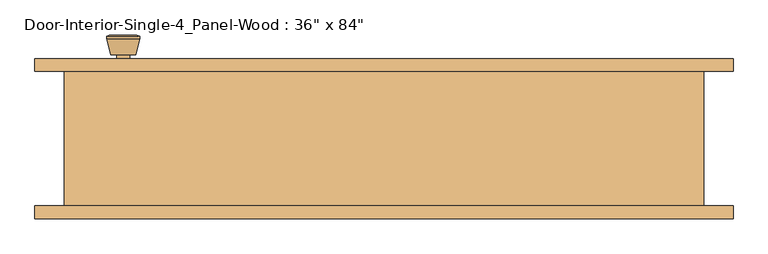
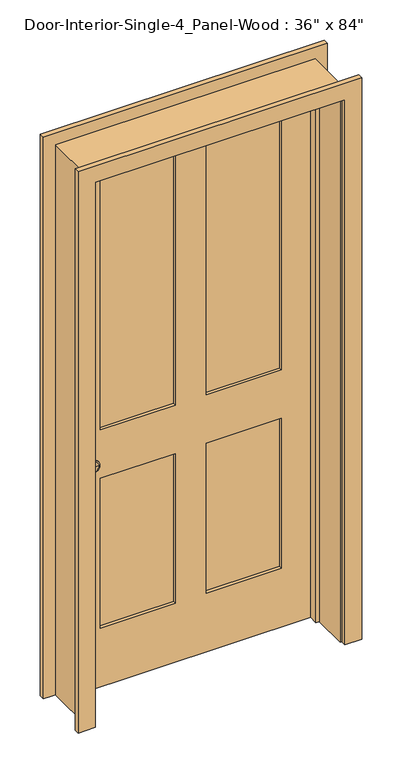
"""IFC4 building model written with IfcOpenShell, lengths in millimetres: door geometry."""

from ifc_helpers import new_model, si_unit, point, frame, frame_2d, origin, place, context, project, spatial, polyline, circle_curve, trimmed, segment, composite_curve, outline, extrude, faceted_brep, source, transform, mapped, element, save
from ifc_brep_helpers import plane_surface, cylinder_surface, revolved_surface, advanced_brep


def door_2d5c49d3(model_context):
    return source(origin(), model_context, "Body", "SolidModel", [
        advanced_brep(
        [(-393.7, 57.5, 914.4), (-383.7, 57.5, 914.4), (-403.7, 57.5, 914.4), (-373.2241324, 8.5, 914.4), (-393.7, 8.5, 914.4), (-414.1758676, 8.5, 914.4), (-368.7, 10.3278681, 914.4), (-418.7, 10.3278681, 914.4), (-368.7, 13.7915463, 914.4), (-418.7, 13.7915463, 914.4), (-375.063764, 38.5, 914.4), (-412.336236, 38.5, 914.4), (-383.7, 38.5, 914.4), (-403.7, 38.5, 914.4)],
        [
            (0, 1),
            (1, 2, circle_curve(frame((-393.7, 57.5, 914.4), z_axis=(0.0, 1.0, 0.0), x_axis=(-1.0, 0.0, 0.0)), 10.0)),
            (2, 0),
            (2, 1, circle_curve(frame((-393.7, 57.5, 914.4), z_axis=(0.0, 1.0, 0.0), x_axis=(-1.0, 0.0, 0.0)), 10.0)),
            (3, 4),
            (4, 5),
            (5, 3, circle_curve(frame((-393.7, 8.5, 914.4), z_axis=(0.0, -1.0, 0.0), x_axis=(-1.0, 0.0, 0.0)), 20.4758676)),
            (3, 5, circle_curve(frame((-393.7, 8.5, 914.4), z_axis=(0.0, -1.0, 0.0), x_axis=(-1.0, 0.0, 0.0)), 20.4758676)),
            (6, 3),
            (5, 7),
            (7, 6, circle_curve(frame((-393.7, 10.3278681, 914.4), z_axis=(0.0, -1.0, 0.0), x_axis=(-1.0, 0.0, 0.0)), 25.0)),
            (6, 7, circle_curve(frame((-393.7, 10.3278681, 914.4), z_axis=(0.0, -1.0, 0.0), x_axis=(-1.0, 0.0, 0.0)), 25.0)),
            (8, 6),
            (7, 9),
            (9, 8, circle_curve(frame((-393.7, 13.7915463, 914.4), z_axis=(0.0, -1.0, 0.0), x_axis=(-1.0, 0.0, 0.0)), 25.0)),
            (8, 9, circle_curve(frame((-393.7, 13.7915463, 914.4), z_axis=(0.0, -1.0, 0.0), x_axis=(-1.0, 0.0, 0.0)), 25.0)),
            (10, 8),
            (9, 11),
            (11, 10, circle_curve(frame((-393.7, 38.5, 914.4), z_axis=(0.0, -1.0, 0.0), x_axis=(-1.0, 0.0, 0.0)), 18.636236)),
            (10, 11, circle_curve(frame((-393.7, 38.5, 914.4), z_axis=(0.0, -1.0, 0.0), x_axis=(-1.0, 0.0, 0.0)), 18.636236)),
            (12, 10),
            (11, 13),
            (13, 12, circle_curve(frame((-393.7, 38.5, 914.4), z_axis=(0.0, -1.0, 0.0), x_axis=(-1.0, 0.0, 0.0)), 10.0)),
            (12, 13, circle_curve(frame((-393.7, 38.5, 914.4), z_axis=(0.0, -1.0, 0.0), x_axis=(-1.0, 0.0, 0.0)), 10.0)),
            (1, 12),
            (13, 2),
        ],
        [
            plane_surface(frame((-393.7, 57.5, 914.4), z_axis=(0.0, 1.0, 0.0), x_axis=(-1.0, 0.0, 0.0))),
            plane_surface(frame((-393.7, 8.5, 914.4), z_axis=(0.0, -1.0, 0.0), x_axis=(-1.0, 0.0, 0.0))),
            revolved_surface(polyline([(-414.1758676, 8.5, 914.4), (-418.7, 10.3278681, 914.4)]), (-393.7, 57.5, 914.4), (0.0, 1.0, 0.0)),
            cylinder_surface(frame((-393.7, 57.5, 914.4), z_axis=(0.0, 1.0, 0.0), x_axis=(-1.0, 0.0, 0.0)), 25.0),
            revolved_surface(polyline([(-418.7, 13.7915463, 914.4), (-412.336236, 38.5, 914.4)]), (-393.7, 57.5, 914.4), (0.0, 1.0, 0.0)),
            plane_surface(frame((-393.7, 38.5, 914.4), z_axis=(0.0, 1.0, 0.0), x_axis=(-1.0, 0.0, 0.0))),
            cylinder_surface(frame((-393.7, 57.5, 914.4), z_axis=(0.0, 1.0, 0.0), x_axis=(-1.0, 0.0, 0.0)), 10.0),
        ],
        [
            (0, [[1, 2, 3]]),
            (0, [[-3, 4, -1]]),
            (1, [[5, 6, 7]]),
            (1, [[-6, -5, 8]]),
            (2, [[9, -7, 10, 11]]),
            (2, [[-10, -8, -9, 12]]),
            (3, [[13, -11, 14, 15]]),
            (3, [[-14, -12, -13, 16]]),
            (4, [[17, -15, 18, 19]]),
            (4, [[-18, -16, -17, 20]]),
            (5, [[21, -19, 22, 23]]),
            (5, [[-22, -20, -21, 24]]),
            (6, [[25, -23, 26, -2]]),
            (6, [[-26, -24, -25, -4]]),
        ],
    ),
        extrude(outline(composite_curve([segment(trimmed(circle_curve(frame_2d((914.4, -393.7)), 30.0), [point((914.4, -423.7))], [point((914.4, -363.7))], False, "CARTESIAN"), True, "CONTINUOUS"), segment(trimmed(circle_curve(frame_2d((914.4, -393.7)), 30.0), [point((914.4, -363.7))], [point((914.4, -423.7))], False, "CARTESIAN"), True, "CONTINUOUS")], self_intersect=False)), frame((0.0, 57.5, 0.0), z_axis=(0.0, 1.0, 0.0), x_axis=(0.0, 0.0, 1.0)), (0.0, 0.0, 1.0), 6.0),
        advanced_brep(
        [(-393.7, 104.425, 914.4), (-403.7, 104.425, 914.4), (-383.7, 104.425, 914.4), (-373.2241324, 153.425, 914.4), (-414.1758676, 153.425, 914.4), (-393.7, 153.425, 914.4), (-368.7, 151.5971319, 914.4), (-418.7, 151.5971319, 914.4), (-368.7, 148.1334537, 914.4), (-418.7, 148.1334537, 914.4), (-375.063764, 123.425, 914.4), (-412.336236, 123.425, 914.4), (-383.7, 123.425, 914.4), (-403.7, 123.425, 914.4)],
        [
            (0, 1),
            (1, 2, circle_curve(frame((-393.7, 104.425, 914.4), z_axis=(0.0, -1.0, 0.0), x_axis=(-1.0, 0.0, 0.0)), 10.0)),
            (2, 0),
            (2, 1, circle_curve(frame((-393.7, 104.425, 914.4), z_axis=(0.0, -1.0, 0.0), x_axis=(-1.0, 0.0, 0.0)), 10.0)),
            (3, 4, circle_curve(frame((-393.7, 153.425, 914.4), z_axis=(0.0, 1.0, 0.0), x_axis=(-1.0, 0.0, 0.0)), 20.4758676)),
            (4, 5),
            (5, 3),
            (4, 3, circle_curve(frame((-393.7, 153.425, 914.4), z_axis=(0.0, 1.0, 0.0), x_axis=(-1.0, 0.0, 0.0)), 20.4758676)),
            (6, 7, circle_curve(frame((-393.7, 151.5971319, 914.4), z_axis=(0.0, 1.0, 0.0), x_axis=(-1.0, 0.0, 0.0)), 25.0)),
            (7, 4),
            (3, 6),
            (7, 6, circle_curve(frame((-393.7, 151.5971319, 914.4), z_axis=(0.0, 1.0, 0.0), x_axis=(-1.0, 0.0, 0.0)), 25.0)),
            (8, 9, circle_curve(frame((-393.7, 148.1334537, 914.4), z_axis=(0.0, 1.0, 0.0), x_axis=(-1.0, 0.0, 0.0)), 25.0)),
            (9, 7),
            (6, 8),
            (9, 8, circle_curve(frame((-393.7, 148.1334537, 914.4), z_axis=(0.0, 1.0, 0.0), x_axis=(-1.0, 0.0, 0.0)), 25.0)),
            (10, 11, circle_curve(frame((-393.7, 123.425, 914.4), z_axis=(0.0, 1.0, 0.0), x_axis=(-1.0, 0.0, 0.0)), 18.636236)),
            (11, 9),
            (8, 10),
            (11, 10, circle_curve(frame((-393.7, 123.425, 914.4), z_axis=(0.0, 1.0, 0.0), x_axis=(-1.0, 0.0, 0.0)), 18.636236)),
            (12, 13, circle_curve(frame((-393.7, 123.425, 914.4), z_axis=(0.0, 1.0, 0.0), x_axis=(-1.0, 0.0, 0.0)), 10.0)),
            (13, 11),
            (10, 12),
            (13, 12, circle_curve(frame((-393.7, 123.425, 914.4), z_axis=(0.0, 1.0, 0.0), x_axis=(-1.0, 0.0, 0.0)), 10.0)),
            (1, 13),
            (12, 2),
        ],
        [
            plane_surface(frame((-393.7, 104.425, 914.4), z_axis=(0.0, -1.0, 0.0), x_axis=(-1.0, 0.0, 0.0))),
            plane_surface(frame((-393.7, 153.425, 914.4), z_axis=(0.0, 1.0, 0.0), x_axis=(-1.0, 0.0, 0.0))),
            revolved_surface(polyline([(-414.1758676, 153.425, 914.4), (-418.7, 151.5971319, 914.4)]), (-393.7, 104.425, 914.4), (0.0, -1.0, 0.0)),
            cylinder_surface(frame((-393.7, 104.425, 914.4), z_axis=(0.0, -1.0, 0.0), x_axis=(-1.0, 0.0, 0.0)), 25.0),
            revolved_surface(polyline([(-418.7, 148.1334537, 914.4), (-412.336236, 123.425, 914.4)]), (-393.7, 104.425, 914.4), (0.0, -1.0, 0.0)),
            plane_surface(frame((-393.7, 123.425, 914.4), z_axis=(0.0, -1.0, 0.0), x_axis=(-1.0, 0.0, 0.0))),
            cylinder_surface(frame((-393.7, 104.425, 914.4), z_axis=(0.0, -1.0, 0.0), x_axis=(-1.0, 0.0, 0.0)), 10.0),
        ],
        [
            (0, [[1, 2, 3]]),
            (0, [[-3, 4, -1]]),
            (1, [[5, 6, 7]]),
            (1, [[8, -7, -6]]),
            (2, [[9, 10, -5, 11]]),
            (2, [[12, -11, -8, -10]]),
            (3, [[13, 14, -9, 15]]),
            (3, [[16, -15, -12, -14]]),
            (4, [[17, 18, -13, 19]]),
            (4, [[20, -19, -16, -18]]),
            (5, [[21, 22, -17, 23]]),
            (5, [[24, -23, -20, -22]]),
            (6, [[-2, 25, -21, 26]]),
            (6, [[-4, -26, -24, -25]]),
        ],
    ),
        extrude(outline(composite_curve([segment(trimmed(circle_curve(frame_2d((914.4, -393.7)), 30.0), [point((914.4, -423.7))], [point((914.4, -363.7))], False, "CARTESIAN"), True, "CONTINUOUS"), segment(trimmed(circle_curve(frame_2d((914.4, -393.7)), 30.0), [point((914.4, -363.7))], [point((914.4, -423.7))], False, "CARTESIAN"), True, "CONTINUOUS")], self_intersect=False)), frame((0.0, 98.425, 0.0), z_axis=(0.0, 1.0, 0.0), x_axis=(0.0, 0.0, 1.0)), (0.0, 0.0, 1.0), 6.0),
        faceted_brep([(482.6, 98.425, 0.0), (482.6, -104.775, 0.0), (457.2, -104.775, 0.0), (457.2, 28.575, 0.0), (444.5, 28.575, 0.0), (444.5, 63.5, 0.0), (457.2, 63.5, 0.0), (457.2, 98.425, 0.0), (482.6, 98.425, 2159.0), (482.6, -104.775, 2159.0), (-482.6, -104.775, 2159.0), (-482.6, -104.775, 0.0), (-457.2, -104.775, 0.0), (-457.2, -104.775, 2133.6), (457.2, -104.775, 2133.6), (457.2, 28.575, 2133.6), (-457.2, 28.575, 2133.6), (-457.2, 28.575, 0.0), (-444.5, 28.575, 0.0), (-444.5, 28.575, 2120.9), (444.5, 28.575, 2120.9), (444.5, 63.5, 2120.9), (-444.5, 63.5, 2120.9), (-444.5, 63.5, 0.0), (-457.2, 63.5, 0.0), (-457.2, 63.5, 2133.6), (457.2, 63.5, 2133.6), (457.2, 98.425, 2133.6), (-457.2, 98.425, 2133.6), (-457.2, 98.425, 0.0), (-482.6, 98.425, 0.0), (-482.6, 98.425, 2159.0)], [[[0, 1, 2, 3, 4, 5, 6, 7]], [[1, 0, 8, 9]], [[2, 1, 9, 10, 11, 12, 13, 14]], [[3, 2, 14, 15]], [[4, 3, 15, 16, 17, 18, 19, 20]], [[5, 4, 20, 21]], [[6, 5, 21, 22, 23, 24, 25, 26]], [[7, 6, 26, 27]], [[0, 7, 27, 28, 29, 30, 31, 8]], [[9, 8, 31, 10]], [[15, 14, 13, 16]], [[21, 20, 19, 22]], [[27, 26, 25, 28]], [[30, 29, 24, 23, 18, 17, 12, 11]], [[10, 31, 30, 11]], [[16, 13, 12, 17]], [[22, 19, 18, 23]], [[28, 25, 24, 29]]]),
        extrude(outline(polyline([(2133.6, -457.2), (0.0, -457.2), (0.0, 457.2), (2133.6, 457.2), (2133.6, -457.2)]), holes=[polyline([(2014.5375, 57.15), (2014.5375, 336.55), (1009.65, 336.55), (1009.65, 57.15), (2014.5375, 57.15)]), polyline([(1009.65, -57.15), (1009.65, -336.55), (2014.5375, -336.55), (2014.5375, -57.15), (1009.65, -57.15)]), polyline([(819.15, 57.15), (819.15, 336.55), (231.775, 336.55), (231.775, 57.15), (819.15, 57.15)]), polyline([(231.775, -57.15), (231.775, -336.55), (819.15, -336.55), (819.15, -57.15), (231.775, -57.15)])]), frame((0.0, 63.5, 0.0), z_axis=(0.0, 1.0, 0.0), x_axis=(0.0, 0.0, 1.0)), (0.0, 0.0, 1.0), 34.925),
        extrude(outline(polyline([(336.55, 75.1416667), (57.15, 75.1416667), (57.15, 86.7833333), (336.55, 86.7833333), (336.55, 75.1416667)])), frame((0.0, 0.0, 1009.65), z_axis=(0.0, 0.0, 1.0), x_axis=(1.0, 0.0, 0.0)), (0.0, 0.0, 1.0), 1004.8875),
        extrude(outline(polyline([(-57.15, 75.1416667), (-336.55, 75.1416667), (-336.55, 86.7833333), (-57.15, 86.7833333), (-57.15, 75.1416667)])), frame((0.0, 0.0, 1009.65), z_axis=(0.0, 0.0, 1.0), x_axis=(1.0, 0.0, 0.0)), (0.0, 0.0, 1.0), 1004.8875),
        extrude(outline(polyline([(336.55, 75.1416667), (57.15, 75.1416667), (57.15, 86.7833333), (336.55, 86.7833333), (336.55, 75.1416667)])), frame((0.0, 0.0, 231.775), z_axis=(0.0, 0.0, 1.0), x_axis=(1.0, 0.0, 0.0)), (0.0, 0.0, 1.0), 587.375),
        extrude(outline(polyline([(-57.15, 75.1416667), (-336.55, 75.1416667), (-336.55, 86.7833333), (-57.15, 86.7833333), (-57.15, 75.1416667)])), frame((0.0, 0.0, 231.775), z_axis=(0.0, 0.0, 1.0), x_axis=(1.0, 0.0, 0.0)), (0.0, 0.0, 1.0), 587.375),
        extrude(outline(polyline([(0.0, 463.55), (0.0, 527.05), (2203.45, 527.05), (2203.45, -527.05), (0.0, -527.05), (0.0, -463.55), (2139.95, -463.55), (2139.95, 463.55), (0.0, 463.55)])), frame((0.0, 98.425, 0.0), z_axis=(0.0, 1.0, 0.0), x_axis=(0.0, 0.0, 1.0)), (0.0, 0.0, 1.0), 19.05),
        extrude(outline(polyline([(0.0, 463.55), (0.0, 527.05), (2203.45, 527.05), (2203.45, -527.05), (0.0, -527.05), (0.0, -463.55), (2139.95, -463.55), (2139.95, 463.55), (0.0, 463.55)])), frame((0.0, -123.825, 0.0), z_axis=(0.0, 1.0, 0.0), x_axis=(0.0, 0.0, 1.0)), (0.0, 0.0, 1.0), 19.05),
    ])


if __name__ == "__main__":
    model = new_model("IFC4")
    model_context = context("Model", 3, world=origin())
    ifc_project = project(units=[si_unit("LENGTHUNIT", "METRE", prefix="MILLI")], contexts=[model_context])
    site = spatial("IfcSite", under=ifc_project)
    building = spatial("IfcBuilding", under=site)
    placement = place(None, origin())
    door_shape = door_2d5c49d3(model_context)
    element("IfcDoor", 1, ObjectType="Door-Interior-Single-4_Panel-Wood : 36\" x 84\"", at=placement, inside=building, context=model_context, shape_type="MappedRepresentation", body=[
        mapped(door_shape, transform((0.0, 0.0, 0.0), x_axis=(1.0, 0.0, 0.0), y_axis=(0.0, 1.0, 0.0), z_axis=(0.0, 0.0, 1.0))),
    ])
    save(model, "model.ifc")

# Revit data of these elements
# Type "Door-Interior-Single-4_Panel-Wood : 36\" x 84\""
#   Type Mark = "8"
#   Assembly Code = "C1020300"
#   Analytic Construction = "Wooden"
#   Top Rail = 0' - 4 11/16"
#   Thickness = 0' - 1 3/8"
#   Thermal Resistance (R) = 2.5876 (h·ft²·°F)/BTU
#   Swing Angle [instance default] = 90.00°
#   Stiles = 0' - 4 3/4"
#   Rough Width = 3' - 2"
#   Rough Height = 7' - 1"
#   Mullion = 0' - 4 1/2"
#   Lock Rail = 0' - 7 1/2"
#   Height = 7' - 0"
#   Width = 3' - 0"
#   Heat Transfer Coefficient (U) = 0.3865 BTU/(h·ft²·°F)
#   Bottom Rail = 0' - 9 1/8"
#   Trim Material = Cherry
#   Panel Material = Cherry
#   Frame Material = Cherry
#   Door Handle Material = Aluminum
#   Visual Light Transmittance = 0
#   Solar Heat Gain Coefficient = 0
#   Wall Closure = (empty or 0)
#   Function = (empty or 0)
# Element 1 (IfcDoor, "Door-Interior-Single-4_Panel-Wood : 36\" x 84\"")
#   Materials on its faces: "Cherry", "Aluminum"
# Materials
#   "Cherry": class "Wood", colour RGB 226 177 128, transparency 0, Description = "Prunus Serotina", Cost = 0
#   "Aluminum": class "Metal", colour RGB 247 247 247, transparency 0, Description = "Aluminum 6061", Cost = 0
